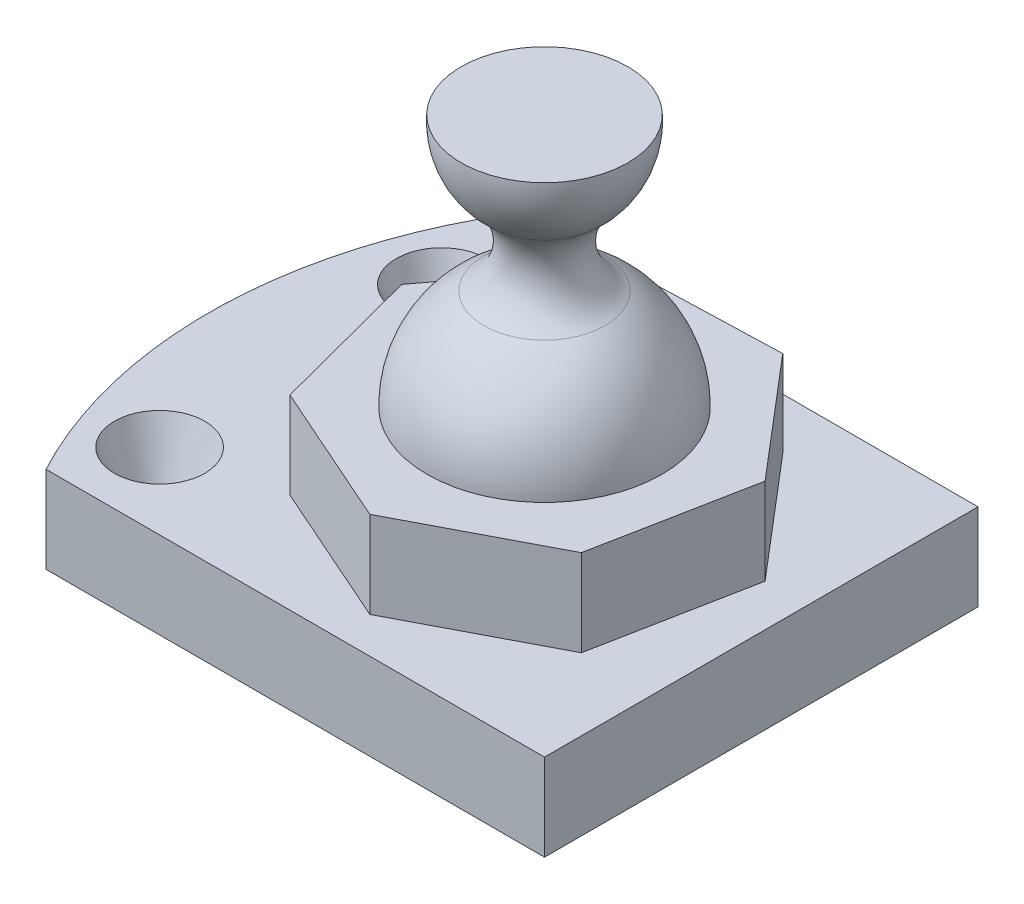
ISO-10303-21;
HEADER;
FILE_DESCRIPTION(('STEP AP214'),'2;1');
FILE_NAME('part.step','',(''),(''),'','','');
FILE_SCHEMA(('AUTOMOTIVE_DESIGN { 1 0 10303 214 1 1 1 1 }'));
ENDSEC;
DATA;
#1=APPLICATION_CONTEXT('core data for automotive mechanical design processes');
#2=APPLICATION_PROTOCOL_DEFINITION('international standard','automotive_design',2000,#1);
#3=PRODUCT_CONTEXT('',#1,'mechanical');
#4=PRODUCT('Part','Part','',(#3));
#5=PRODUCT_RELATED_PRODUCT_CATEGORY('part','',(#4));
#6=PRODUCT_DEFINITION_FORMATION('','',#4);
#7=PRODUCT_DEFINITION_CONTEXT('part definition',#1,'design');
#8=PRODUCT_DEFINITION('design','',#6,#7);
#9=PRODUCT_DEFINITION_SHAPE('','',#8);
#10=(LENGTH_UNIT() NAMED_UNIT(*) SI_UNIT(.MILLI.,.METRE.));
#11=(NAMED_UNIT(*) PLANE_ANGLE_UNIT() SI_UNIT($,.RADIAN.));
#12=(NAMED_UNIT(*) SI_UNIT($,.STERADIAN.) SOLID_ANGLE_UNIT());
#13=UNCERTAINTY_MEASURE_WITH_UNIT(LENGTH_MEASURE(1.E-05),#10,'distance_accuracy_value','');
#14=(GEOMETRIC_REPRESENTATION_CONTEXT(3) GLOBAL_UNCERTAINTY_ASSIGNED_CONTEXT((#13)) GLOBAL_UNIT_ASSIGNED_CONTEXT((#10,
#11,#12)) REPRESENTATION_CONTEXT('',''));
#15=CARTESIAN_POINT('',(0.,0.,0.));
#16=DIRECTION('',(0.,0.,1.));
#17=DIRECTION('',(1.,0.,0.));
#18=AXIS2_PLACEMENT_3D('',#15,#16,#17);
#19=CARTESIAN_POINT('',(0.,0.,0.));
#20=DIRECTION('',(0.,-1.,0.));
#21=DIRECTION('',(1.,0.,0.));
#22=AXIS2_PLACEMENT_3D('',#19,#20,#21);
#23=SPHERICAL_SURFACE('',#22,32.4762304839796);
#24=CARTESIAN_POINT('',(0.,27.8110758941161,0.));
#25=DIRECTION('',(0.,-1.,0.));
#26=DIRECTION('',(0.,0.,-1.));
#27=AXIS2_PLACEMENT_3D('',#24,#25,#26);
#28=CIRCLE('',#27,16.7704980266027);
#29=CARTESIAN_POINT('',(0.,27.8110758941161,-16.7704980266027));
#30=VERTEX_POINT('',#29);
#31=EDGE_CURVE('E172',#30,#30,#28,.T.);
#32=ORIENTED_EDGE('',*,*,#31,.T.);
#33=EDGE_LOOP('',(#32));
#34=FACE_BOUND('',#33,.T.);
#35=CARTESIAN_POINT('',(0.,0.,0.));
#36=DIRECTION('',(0.,-1.,0.));
#37=DIRECTION('',(0.,0.,-1.));
#38=AXIS2_PLACEMENT_3D('',#35,#36,#37);
#39=CIRCLE('',#38,32.4762304839796);
#40=CARTESIAN_POINT('',(0.,0.,-32.4762304839796));
#41=VERTEX_POINT('',#40);
#42=EDGE_CURVE('E49',#41,#41,#39,.T.);
#43=ORIENTED_EDGE('',*,*,#42,.F.);
#44=EDGE_LOOP('',(#43));
#45=FACE_BOUND('',#44,.T.);
#46=ADVANCED_FACE('F37',(#34,#45),#23,.T.);
#47=CARTESIAN_POINT('',(0.,39.8,0.));
#48=DIRECTION('',(0.,-1.,0.));
#49=DIRECTION('',(0.,0.,-1.));
#50=AXIS2_PLACEMENT_3D('',#47,#48,#49);
#51=TOROIDAL_SURFACE('',#50,24.,14.);
#52=CARTESIAN_POINT('',(0.,50.3791238896694,0.));
#53=DIRECTION('',(0.,-1.,0.));
#54=DIRECTION('',(0.,0.,-1.));
#55=AXIS2_PLACEMENT_3D('',#52,#53,#54);
#56=CIRCLE('',#55,14.8303687245873);
#57=CARTESIAN_POINT('',(0.,50.3791238896694,-14.8303687245873));
#58=VERTEX_POINT('',#57);
#59=EDGE_CURVE('E168',#58,#58,#56,.T.);
#60=ORIENTED_EDGE('',*,*,#59,.T.);
#61=EDGE_LOOP('',(#60));
#62=FACE_BOUND('',#61,.T.);
#63=ORIENTED_EDGE('',*,*,#31,.F.);
#64=EDGE_LOOP('',(#63));
#65=FACE_BOUND('',#64,.T.);
#66=ADVANCED_FACE('F185',(#62,#65),#51,.F.);
#67=CARTESIAN_POINT('',(0.,68.5147648433883,0.));
#68=DIRECTION('',(0.,-1.,0.));
#69=DIRECTION('',(0.,0.,-1.));
#70=AXIS2_PLACEMENT_3D('',#67,#68,#69);
#71=DEGENERATE_TOROIDAL_SURFACE('',#70,0.888999176120141,24.,.F.);
#72=CARTESIAN_POINT('',(0.,70.,0.));
#73=DIRECTION('',(0.,-1.,0.));
#74=DIRECTION('',(0.,0.,-1.));
#75=AXIS2_PLACEMENT_3D('',#72,#73,#74);
#76=CIRCLE('',#75,23.065);
#77=CARTESIAN_POINT('',(0.,70.,-23.065));
#78=VERTEX_POINT('',#77);
#79=EDGE_CURVE('E170',#78,#78,#76,.T.);
#80=ORIENTED_EDGE('',*,*,#79,.T.);
#81=EDGE_LOOP('',(#80));
#82=FACE_BOUND('',#81,.T.);
#83=ORIENTED_EDGE('',*,*,#59,.F.);
#84=EDGE_LOOP('',(#83));
#85=FACE_BOUND('',#84,.T.);
#86=ADVANCED_FACE('F189',(#82,#85),#71,.F.);
#87=CARTESIAN_POINT('',(0.,70.,0.));
#88=DIRECTION('',(0.,1.,0.));
#89=DIRECTION('',(0.,0.,1.));
#90=AXIS2_PLACEMENT_3D('',#87,#88,#89);
#91=PLANE('',#90);
#92=ORIENTED_EDGE('',*,*,#79,.F.);
#93=EDGE_LOOP('',(#92));
#94=FACE_BOUND('',#93,.T.);
#95=ADVANCED_FACE('F195',(#94),#91,.T.);
#96=CARTESIAN_POINT('',(0.,0.,0.));
#97=DIRECTION('',(0.,-1.,0.));
#98=DIRECTION('',(0.,0.,-1.));
#99=AXIS2_PLACEMENT_3D('',#96,#97,#98);
#100=PLANE('',#99);
#101=ORIENTED_EDGE('',*,*,#42,.T.);
#102=EDGE_LOOP('',(#101));
#103=FACE_BOUND('',#102,.T.);
#104=DIRECTION('',(-0.886439698937166,0.,0.462844099182637));
#105=VECTOR('',#104,1.);
#106=CARTESIAN_POINT('',(40.0809947566498,0.,29.8917021816659));
#107=LINE('',#106,#105);
#108=CARTESIAN_POINT('',(40.0809947566498,0.,29.8917021816659));
#109=VERTEX_POINT('',#108);
#110=CARTESIAN_POINT('',(1.61981764893979,0.,49.973755019852));
#111=VERTEX_POINT('',#110);
#112=EDGE_CURVE('E145',#109,#111,#107,.T.);
#113=ORIENTED_EDGE('',*,*,#112,.F.);
#114=DIRECTION('',(-0.190820024034508,0.,0.981625039629425));
#115=VECTOR('',#114,1.);
#116=CARTESIAN_POINT('',(48.3603653093092,0.,-12.6994120789177));
#117=LINE('',#116,#115);
#118=CARTESIAN_POINT('',(48.3603653093092,0.,-12.6994120789177));
#119=VERTEX_POINT('',#118);
#120=EDGE_CURVE('E90',#119,#109,#117,.T.);
#121=ORIENTED_EDGE('',*,*,#120,.F.);
#122=DIRECTION('',(0.648491020985258,0.,0.761222303733606));
#123=VECTOR('',#122,1.);
#124=CARTESIAN_POINT('',(20.2233944123846,0.,-45.7276100232795));
#125=LINE('',#124,#123);
#126=CARTESIAN_POINT('',(20.2233944123846,0.,-45.7276100232795));
#127=VERTEX_POINT('',#126);
#128=EDGE_CURVE('E85',#127,#119,#125,.T.);
#129=ORIENTED_EDGE('',*,*,#128,.F.);
#130=DIRECTION('',(0.99947510039704,0.,-0.0323963529787958));
#131=VECTOR('',#130,1.);
#132=CARTESIAN_POINT('',(-23.1422049591319,0.,-44.3219849468583));
#133=LINE('',#132,#131);
#134=CARTESIAN_POINT('',(-23.1422049591319,0.,-44.3219849468583));
#135=VERTEX_POINT('',#134);
#136=EDGE_CURVE('E153',#135,#127,#133,.T.);
#137=ORIENTED_EDGE('',*,*,#136,.F.);
#138=DIRECTION('',(0.597834043633319,0.,-0.801619895132996));
#139=VECTOR('',#138,1.);
#140=CARTESIAN_POINT('',(-49.0812519814712,0.,-9.54100120172539));
#141=LINE('',#140,#139);
#142=CARTESIAN_POINT('',(-49.0812519814712,0.,-9.54100120172539));
#143=VERTEX_POINT('',#142);
#144=EDGE_CURVE('E117',#143,#135,#141,.T.);
#145=ORIENTED_EDGE('',*,*,#144,.F.);
#146=DIRECTION('',(-0.253988241578353,0.,-0.967207306186185));
#147=VECTOR('',#146,1.);
#148=CARTESIAN_POINT('',(-38.0611151866803,0.,32.4245510492629));
#149=LINE('',#148,#147);
#150=CARTESIAN_POINT('',(-38.0611151866803,0.,32.4245510492629));
#151=VERTEX_POINT('',#150);
#152=EDGE_CURVE('E147',#151,#143,#149,.T.);
#153=ORIENTED_EDGE('',*,*,#152,.F.);
#154=DIRECTION('',(-0.91455220046559,0.,-0.404467888247692));
#155=VECTOR('',#154,1.);
#156=CARTESIAN_POINT('',(1.61981764893979,0.,49.973755019852));
#157=LINE('',#156,#155);
#158=EDGE_CURVE('E150',#111,#151,#157,.T.);
#159=ORIENTED_EDGE('',*,*,#158,.F.);
#160=EDGE_LOOP('',(#113,#121,#129,#137,#145,#153,#159));
#161=FACE_BOUND('',#160,.T.);
#162=ADVANCED_FACE('F180',(#103,#161),#100,.F.);
#163=CARTESIAN_POINT('',(40.0809947566498,-24.,29.8917021816659));
#164=DIRECTION('',(-0.462844099182637,0.,-0.886439698937166));
#165=DIRECTION('',(-0.886439698937166,0.,0.462844099182637));
#166=AXIS2_PLACEMENT_3D('',#163,#164,#165);
#167=PLANE('',#166);
#168=ORIENTED_EDGE('',*,*,#112,.T.);
#169=DIRECTION('',(0.,1.,0.));
#170=VECTOR('',#169,1.);
#171=CARTESIAN_POINT('',(1.61981764893979,-24.,49.973755019852));
#172=LINE('',#171,#170);
#173=CARTESIAN_POINT('',(1.61981764893979,-24.,49.973755019852));
#174=VERTEX_POINT('',#173);
#175=EDGE_CURVE('E164',#174,#111,#172,.T.);
#176=ORIENTED_EDGE('',*,*,#175,.F.);
#177=DIRECTION('',(-0.886439698937166,0.,0.462844099182637));
#178=VECTOR('',#177,1.);
#179=CARTESIAN_POINT('',(40.0809947566498,-24.,29.8917021816659));
#180=LINE('',#179,#178);
#181=CARTESIAN_POINT('',(40.0809947566498,-24.,29.8917021816659));
#182=VERTEX_POINT('',#181);
#183=EDGE_CURVE('E160',#182,#174,#180,.T.);
#184=ORIENTED_EDGE('',*,*,#183,.F.);
#185=DIRECTION('',(0.,1.,0.));
#186=VECTOR('',#185,1.);
#187=CARTESIAN_POINT('',(40.0809947566498,-24.,29.8917021816659));
#188=LINE('',#187,#186);
#189=EDGE_CURVE('E141',#182,#109,#188,.T.);
#190=ORIENTED_EDGE('',*,*,#189,.T.);
#191=EDGE_LOOP('',(#168,#176,#184,#190));
#192=FACE_BOUND('',#191,.T.);
#193=ADVANCED_FACE('F196',(#192),#167,.F.);
#194=CARTESIAN_POINT('',(1.61981764893979,-24.,49.973755019852));
#195=DIRECTION('',(0.404467888247692,0.,-0.91455220046559));
#196=DIRECTION('',(-0.91455220046559,0.,-0.404467888247692));
#197=AXIS2_PLACEMENT_3D('',#194,#195,#196);
#198=PLANE('',#197);
#199=ORIENTED_EDGE('',*,*,#158,.T.);
#200=DIRECTION('',(0.,1.,0.));
#201=VECTOR('',#200,1.);
#202=CARTESIAN_POINT('',(-38.0611151866803,-24.,32.4245510492629));
#203=LINE('',#202,#201);
#204=CARTESIAN_POINT('',(-38.0611151866803,-24.,32.4245510492629));
#205=VERTEX_POINT('',#204);
#206=EDGE_CURVE('E165',#205,#151,#203,.T.);
#207=ORIENTED_EDGE('',*,*,#206,.F.);
#208=DIRECTION('',(-0.91455220046559,0.,-0.404467888247692));
#209=VECTOR('',#208,1.);
#210=CARTESIAN_POINT('',(1.61981764893979,-24.,49.973755019852));
#211=LINE('',#210,#209);
#212=EDGE_CURVE('E98',#174,#205,#211,.T.);
#213=ORIENTED_EDGE('',*,*,#212,.F.);
#214=ORIENTED_EDGE('',*,*,#175,.T.);
#215=EDGE_LOOP('',(#199,#207,#213,#214));
#216=FACE_BOUND('',#215,.T.);
#217=ADVANCED_FACE('F203',(#216),#198,.F.);
#218=CARTESIAN_POINT('',(-38.0611151866803,-24.,32.4245510492629));
#219=DIRECTION('',(0.967207306186185,0.,-0.253988241578353));
#220=DIRECTION('',(-0.253988241578353,0.,-0.967207306186185));
#221=AXIS2_PLACEMENT_3D('',#218,#219,#220);
#222=PLANE('',#221);
#223=ORIENTED_EDGE('',*,*,#152,.T.);
#224=DIRECTION('',(0.,1.,0.));
#225=VECTOR('',#224,1.);
#226=CARTESIAN_POINT('',(-49.0812519814712,-24.,-9.54100120172539));
#227=LINE('',#226,#225);
#228=CARTESIAN_POINT('',(-49.0812519814712,-24.,-9.54100120172539));
#229=VERTEX_POINT('',#228);
#230=EDGE_CURVE('E124',#229,#143,#227,.T.);
#231=ORIENTED_EDGE('',*,*,#230,.F.);
#232=DIRECTION('',(-0.253988241578353,0.,-0.967207306186185));
#233=VECTOR('',#232,1.);
#234=CARTESIAN_POINT('',(-38.0611151866803,-24.,32.4245510492629));
#235=LINE('',#234,#233);
#236=EDGE_CURVE('E131',#205,#229,#235,.T.);
#237=ORIENTED_EDGE('',*,*,#236,.F.);
#238=ORIENTED_EDGE('',*,*,#206,.T.);
#239=EDGE_LOOP('',(#223,#231,#237,#238));
#240=FACE_BOUND('',#239,.T.);
#241=ADVANCED_FACE('F202',(#240),#222,.F.);
#242=CARTESIAN_POINT('',(-49.0812519814712,-24.,-9.54100120172539));
#243=DIRECTION('',(0.801619895132996,0.,0.597834043633319));
#244=DIRECTION('',(0.597834043633319,0.,-0.801619895132996));
#245=AXIS2_PLACEMENT_3D('',#242,#243,#244);
#246=PLANE('',#245);
#247=ORIENTED_EDGE('',*,*,#144,.T.);
#248=DIRECTION('',(0.,1.,0.));
#249=VECTOR('',#248,1.);
#250=CARTESIAN_POINT('',(-23.1422049591319,-24.,-44.3219849468583));
#251=LINE('',#250,#249);
#252=CARTESIAN_POINT('',(-23.1422049591319,-24.,-44.3219849468583));
#253=VERTEX_POINT('',#252);
#254=EDGE_CURVE('E109',#253,#135,#251,.T.);
#255=ORIENTED_EDGE('',*,*,#254,.F.);
#256=DIRECTION('',(0.597834043633319,0.,-0.801619895132996));
#257=VECTOR('',#256,1.);
#258=CARTESIAN_POINT('',(-49.0812519814712,-24.,-9.54100120172539));
#259=LINE('',#258,#257);
#260=EDGE_CURVE('E113',#229,#253,#259,.T.);
#261=ORIENTED_EDGE('',*,*,#260,.F.);
#262=ORIENTED_EDGE('',*,*,#230,.T.);
#263=EDGE_LOOP('',(#247,#255,#261,#262));
#264=FACE_BOUND('',#263,.T.);
#265=ADVANCED_FACE('F115',(#264),#246,.F.);
#266=CARTESIAN_POINT('',(-23.1422049591319,-24.,-44.3219849468583));
#267=DIRECTION('',(0.0323963529787958,0.,0.99947510039704));
#268=DIRECTION('',(0.99947510039704,0.,-0.0323963529787958));
#269=AXIS2_PLACEMENT_3D('',#266,#267,#268);
#270=PLANE('',#269);
#271=ORIENTED_EDGE('',*,*,#136,.T.);
#272=DIRECTION('',(0.,1.,0.));
#273=VECTOR('',#272,1.);
#274=CARTESIAN_POINT('',(20.2233944123846,-24.,-45.7276100232795));
#275=LINE('',#274,#273);
#276=CARTESIAN_POINT('',(20.2233944123846,-24.,-45.7276100232795));
#277=VERTEX_POINT('',#276);
#278=EDGE_CURVE('E121',#277,#127,#275,.T.);
#279=ORIENTED_EDGE('',*,*,#278,.F.);
#280=DIRECTION('',(0.99947510039704,0.,-0.0323963529787958));
#281=VECTOR('',#280,1.);
#282=CARTESIAN_POINT('',(-23.1422049591319,-24.,-44.3219849468583));
#283=LINE('',#282,#281);
#284=EDGE_CURVE('E122',#253,#277,#283,.T.);
#285=ORIENTED_EDGE('',*,*,#284,.F.);
#286=ORIENTED_EDGE('',*,*,#254,.T.);
#287=EDGE_LOOP('',(#271,#279,#285,#286));
#288=FACE_BOUND('',#287,.T.);
#289=ADVANCED_FACE('F127',(#288),#270,.F.);
#290=CARTESIAN_POINT('',(20.2233944123846,-24.,-45.7276100232795));
#291=DIRECTION('',(-0.761222303733606,0.,0.648491020985258));
#292=DIRECTION('',(0.648491020985258,0.,0.761222303733606));
#293=AXIS2_PLACEMENT_3D('',#290,#291,#292);
#294=PLANE('',#293);
#295=ORIENTED_EDGE('',*,*,#128,.T.);
#296=DIRECTION('',(0.,1.,0.));
#297=VECTOR('',#296,1.);
#298=CARTESIAN_POINT('',(48.3603653093092,-24.,-12.6994120789177));
#299=LINE('',#298,#297);
#300=CARTESIAN_POINT('',(48.3603653093092,-24.,-12.6994120789177));
#301=VERTEX_POINT('',#300);
#302=EDGE_CURVE('E59',#301,#119,#299,.T.);
#303=ORIENTED_EDGE('',*,*,#302,.F.);
#304=DIRECTION('',(0.648491020985258,0.,0.761222303733606));
#305=VECTOR('',#304,1.);
#306=CARTESIAN_POINT('',(20.2233944123846,-24.,-45.7276100232795));
#307=LINE('',#306,#305);
#308=EDGE_CURVE('E129',#277,#301,#307,.T.);
#309=ORIENTED_EDGE('',*,*,#308,.F.);
#310=ORIENTED_EDGE('',*,*,#278,.T.);
#311=EDGE_LOOP('',(#295,#303,#309,#310));
#312=FACE_BOUND('',#311,.T.);
#313=ADVANCED_FACE('F213',(#312),#294,.F.);
#314=CARTESIAN_POINT('',(48.3603653093092,-24.,-12.6994120789177));
#315=DIRECTION('',(-0.981625039629425,0.,-0.190820024034508));
#316=DIRECTION('',(-0.190820024034508,0.,0.981625039629425));
#317=AXIS2_PLACEMENT_3D('',#314,#315,#316);
#318=PLANE('',#317);
#319=ORIENTED_EDGE('',*,*,#120,.T.);
#320=ORIENTED_EDGE('',*,*,#189,.F.);
#321=DIRECTION('',(-0.190820024034508,0.,0.981625039629425));
#322=VECTOR('',#321,1.);
#323=CARTESIAN_POINT('',(48.3603653093092,-24.,-12.6994120789177));
#324=LINE('',#323,#322);
#325=EDGE_CURVE('E143',#301,#182,#324,.T.);
#326=ORIENTED_EDGE('',*,*,#325,.F.);
#327=ORIENTED_EDGE('',*,*,#302,.T.);
#328=EDGE_LOOP('',(#319,#320,#326,#327));
#329=FACE_BOUND('',#328,.T.);
#330=ADVANCED_FACE('F216',(#329),#318,.F.);
#331=CARTESIAN_POINT('',(60.,-48.,60.));
#332=DIRECTION('',(-1.,0.,0.));
#333=DIRECTION('',(0.,0.,1.));
#334=AXIS2_PLACEMENT_3D('',#331,#332,#333);
#335=PLANE('',#334);
#336=DIRECTION('',(0.,0.,1.));
#337=VECTOR('',#336,1.);
#338=CARTESIAN_POINT('',(60.,-24.,60.));
#339=LINE('',#338,#337);
#340=CARTESIAN_POINT('',(60.,-24.,-60.));
#341=VERTEX_POINT('',#340);
#342=CARTESIAN_POINT('',(60.,-24.,60.));
#343=VERTEX_POINT('',#342);
#344=EDGE_CURVE('E268',#341,#343,#339,.T.);
#345=ORIENTED_EDGE('',*,*,#344,.T.);
#346=DIRECTION('',(0.,1.,0.));
#347=VECTOR('',#346,1.);
#348=CARTESIAN_POINT('',(60.,-48.,60.));
#349=LINE('',#348,#347);
#350=CARTESIAN_POINT('',(60.,-48.,60.));
#351=VERTEX_POINT('',#350);
#352=EDGE_CURVE('E306',#351,#343,#349,.T.);
#353=ORIENTED_EDGE('',*,*,#352,.F.);
#354=DIRECTION('',(0.,0.,1.));
#355=VECTOR('',#354,1.);
#356=CARTESIAN_POINT('',(60.,-48.,60.));
#357=LINE('',#356,#355);
#358=CARTESIAN_POINT('',(60.,-48.,-60.));
#359=VERTEX_POINT('',#358);
#360=EDGE_CURVE('E277',#359,#351,#357,.T.);
#361=ORIENTED_EDGE('',*,*,#360,.F.);
#362=DIRECTION('',(0.,1.,0.));
#363=VECTOR('',#362,1.);
#364=CARTESIAN_POINT('',(60.,-48.,-60.));
#365=LINE('',#364,#363);
#366=EDGE_CURVE('E288',#359,#341,#365,.T.);
#367=ORIENTED_EDGE('',*,*,#366,.T.);
#368=EDGE_LOOP('',(#345,#353,#361,#367));
#369=FACE_BOUND('',#368,.T.);
#370=ADVANCED_FACE('F218',(#369),#335,.F.);
#371=CARTESIAN_POINT('',(-78.,-48.,60.));
#372=DIRECTION('',(0.,0.,-1.));
#373=DIRECTION('',(-1.,0.,0.));
#374=AXIS2_PLACEMENT_3D('',#371,#372,#373);
#375=PLANE('',#374);
#376=DIRECTION('',(-1.,0.,0.));
#377=VECTOR('',#376,1.);
#378=CARTESIAN_POINT('',(-78.,-24.,60.));
#379=LINE('',#378,#377);
#380=CARTESIAN_POINT('',(-78.,-24.,60.));
#381=VERTEX_POINT('',#380);
#382=EDGE_CURVE('E295',#343,#381,#379,.T.);
#383=ORIENTED_EDGE('',*,*,#382,.T.);
#384=DIRECTION('',(0.,1.,0.));
#385=VECTOR('',#384,1.);
#386=CARTESIAN_POINT('',(-78.,-48.,60.));
#387=LINE('',#386,#385);
#388=CARTESIAN_POINT('',(-78.,-48.,60.));
#389=VERTEX_POINT('',#388);
#390=EDGE_CURVE('E302',#389,#381,#387,.T.);
#391=ORIENTED_EDGE('',*,*,#390,.F.);
#392=DIRECTION('',(-1.,0.,0.));
#393=VECTOR('',#392,1.);
#394=CARTESIAN_POINT('',(-78.,-48.,60.));
#395=LINE('',#394,#393);
#396=EDGE_CURVE('E276',#351,#389,#395,.T.);
#397=ORIENTED_EDGE('',*,*,#396,.F.);
#398=ORIENTED_EDGE('',*,*,#352,.T.);
#399=EDGE_LOOP('',(#383,#391,#397,#398));
#400=FACE_BOUND('',#399,.T.);
#401=ADVANCED_FACE('F226',(#400),#375,.F.);
#402=CARTESIAN_POINT('',(34.5,-48.,0.));
#403=DIRECTION('',(0.,1.,0.));
#404=DIRECTION('',(0.,0.,1.));
#405=AXIS2_PLACEMENT_3D('',#402,#403,#404);
#406=CYLINDRICAL_SURFACE('',#405,127.5);
#407=CARTESIAN_POINT('',(34.5,-24.,0.));
#408=DIRECTION('',(0.,-1.,0.));
#409=DIRECTION('',(0.,0.,1.));
#410=AXIS2_PLACEMENT_3D('',#407,#408,#409);
#411=CIRCLE('',#410,127.5);
#412=CARTESIAN_POINT('',(-78.,-24.,-60.));
#413=VERTEX_POINT('',#412);
#414=EDGE_CURVE('E293',#381,#413,#411,.T.);
#415=ORIENTED_EDGE('',*,*,#414,.T.);
#416=DIRECTION('',(0.,1.,0.));
#417=VECTOR('',#416,1.);
#418=CARTESIAN_POINT('',(-78.,-48.,-60.));
#419=LINE('',#418,#417);
#420=CARTESIAN_POINT('',(-78.,-48.,-60.));
#421=VERTEX_POINT('',#420);
#422=EDGE_CURVE('E301',#421,#413,#419,.T.);
#423=ORIENTED_EDGE('',*,*,#422,.F.);
#424=CARTESIAN_POINT('',(34.5,-48.,0.));
#425=DIRECTION('',(0.,-1.,0.));
#426=DIRECTION('',(0.,0.,1.));
#427=AXIS2_PLACEMENT_3D('',#424,#425,#426);
#428=CIRCLE('',#427,127.5);
#429=EDGE_CURVE('E282',#389,#421,#428,.T.);
#430=ORIENTED_EDGE('',*,*,#429,.F.);
#431=ORIENTED_EDGE('',*,*,#390,.T.);
#432=EDGE_LOOP('',(#415,#423,#430,#431));
#433=FACE_BOUND('',#432,.T.);
#434=ADVANCED_FACE('F233',(#433),#406,.T.);
#435=CARTESIAN_POINT('',(60.,-48.,-60.));
#436=DIRECTION('',(0.,0.,1.));
#437=DIRECTION('',(1.,0.,0.));
#438=AXIS2_PLACEMENT_3D('',#435,#436,#437);
#439=PLANE('',#438);
#440=DIRECTION('',(1.,0.,0.));
#441=VECTOR('',#440,1.);
#442=CARTESIAN_POINT('',(60.,-24.,-60.));
#443=LINE('',#442,#441);
#444=EDGE_CURVE('E278',#413,#341,#443,.T.);
#445=ORIENTED_EDGE('',*,*,#444,.T.);
#446=ORIENTED_EDGE('',*,*,#366,.F.);
#447=DIRECTION('',(1.,0.,0.));
#448=VECTOR('',#447,1.);
#449=CARTESIAN_POINT('',(60.,-48.,-60.));
#450=LINE('',#449,#448);
#451=EDGE_CURVE('E289',#421,#359,#450,.T.);
#452=ORIENTED_EDGE('',*,*,#451,.F.);
#453=ORIENTED_EDGE('',*,*,#422,.T.);
#454=EDGE_LOOP('',(#445,#446,#452,#453));
#455=FACE_BOUND('',#454,.T.);
#456=ADVANCED_FACE('F236',(#455),#439,.F.);
#457=CARTESIAN_POINT('',(34.5,-48.,0.));
#458=DIRECTION('',(0.,1.,0.));
#459=DIRECTION('',(0.,0.,1.));
#460=AXIS2_PLACEMENT_3D('',#457,#458,#459);
#461=PLANE('',#460);
#462=CARTESIAN_POINT('',(-67.55,-48.,-39.));
#463=DIRECTION('',(0.,1.,0.));
#464=DIRECTION('',(0.,0.,1.));
#465=AXIS2_PLACEMENT_3D('',#462,#463,#464);
#466=CIRCLE('',#465,3.76471437761112);
#467=CARTESIAN_POINT('',(-67.55,-48.,-35.2352856223889));
#468=VERTEX_POINT('',#467);
#469=EDGE_CURVE('E265',#468,#468,#466,.F.);
#470=ORIENTED_EDGE('',*,*,#469,.F.);
#471=EDGE_LOOP('',(#470));
#472=FACE_BOUND('',#471,.T.);
#473=CARTESIAN_POINT('',(-67.55,-48.,39.));
#474=DIRECTION('',(0.,1.,0.));
#475=DIRECTION('',(0.,0.,1.));
#476=AXIS2_PLACEMENT_3D('',#473,#474,#475);
#477=CIRCLE('',#476,3.76471437761112);
#478=CARTESIAN_POINT('',(-67.55,-48.,42.7647143776111));
#479=VERTEX_POINT('',#478);
#480=EDGE_CURVE('E271',#479,#479,#477,.F.);
#481=ORIENTED_EDGE('',*,*,#480,.F.);
#482=EDGE_LOOP('',(#481));
#483=FACE_BOUND('',#482,.T.);
#484=ORIENTED_EDGE('',*,*,#360,.T.);
#485=ORIENTED_EDGE('',*,*,#396,.T.);
#486=ORIENTED_EDGE('',*,*,#429,.T.);
#487=ORIENTED_EDGE('',*,*,#451,.T.);
#488=EDGE_LOOP('',(#484,#485,#486,#487));
#489=FACE_BOUND('',#488,.T.);
#490=ADVANCED_FACE('F244',(#472,#483,#489),#461,.F.);
#491=CARTESIAN_POINT('',(34.5,-24.,0.));
#492=DIRECTION('',(0.,1.,0.));
#493=DIRECTION('',(0.,0.,1.));
#494=AXIS2_PLACEMENT_3D('',#491,#492,#493);
#495=PLANE('',#494);
#496=CARTESIAN_POINT('',(-67.55,-24.,-39.));
#497=DIRECTION('',(0.,1.,0.));
#498=DIRECTION('',(0.,0.,1.));
#499=AXIS2_PLACEMENT_3D('',#496,#497,#498);
#500=CIRCLE('',#499,12.5);
#501=CARTESIAN_POINT('',(-67.55,-24.,-26.5));
#502=VERTEX_POINT('',#501);
#503=EDGE_CURVE('E264',#502,#502,#500,.T.);
#504=ORIENTED_EDGE('',*,*,#503,.F.);
#505=EDGE_LOOP('',(#504));
#506=FACE_BOUND('',#505,.T.);
#507=CARTESIAN_POINT('',(-67.55,-24.,39.));
#508=DIRECTION('',(0.,1.,0.));
#509=DIRECTION('',(0.,0.,1.));
#510=AXIS2_PLACEMENT_3D('',#507,#508,#509);
#511=CIRCLE('',#510,12.5);
#512=CARTESIAN_POINT('',(-67.55,-24.,51.5));
#513=VERTEX_POINT('',#512);
#514=EDGE_CURVE('E266',#513,#513,#511,.T.);
#515=ORIENTED_EDGE('',*,*,#514,.F.);
#516=EDGE_LOOP('',(#515));
#517=FACE_BOUND('',#516,.T.);
#518=ORIENTED_EDGE('',*,*,#325,.T.);
#519=ORIENTED_EDGE('',*,*,#183,.T.);
#520=ORIENTED_EDGE('',*,*,#212,.T.);
#521=ORIENTED_EDGE('',*,*,#236,.T.);
#522=ORIENTED_EDGE('',*,*,#260,.T.);
#523=ORIENTED_EDGE('',*,*,#284,.T.);
#524=ORIENTED_EDGE('',*,*,#308,.T.);
#525=EDGE_LOOP('',(#518,#519,#520,#521,#522,#523,#524));
#526=FACE_BOUND('',#525,.T.);
#527=ORIENTED_EDGE('',*,*,#344,.F.);
#528=ORIENTED_EDGE('',*,*,#444,.F.);
#529=ORIENTED_EDGE('',*,*,#414,.F.);
#530=ORIENTED_EDGE('',*,*,#382,.F.);
#531=EDGE_LOOP('',(#527,#528,#529,#530));
#532=FACE_BOUND('',#531,.T.);
#533=ADVANCED_FACE('F134',(#506,#517,#526,#532),#495,.T.);
#534=CARTESIAN_POINT('',(-67.55,-24.,39.));
#535=DIRECTION('',(0.,1.,0.));
#536=DIRECTION('',(0.,0.,1.));
#537=AXIS2_PLACEMENT_3D('',#534,#535,#536);
#538=CONICAL_SURFACE('',#537,12.5,0.349065850398867);
#539=CARTESIAN_POINT('',(-67.55,-48.,42.7647143776111));
#540=CARTESIAN_POINT('',(-67.55,-47.75,42.8557069361777));
#541=CARTESIAN_POINT('',(-67.55,-47.5,42.9466994947442));
#542=CARTESIAN_POINT('',(-67.55,-47.,43.1286846118773));
#543=CARTESIAN_POINT('',(-67.55,-46.75,43.2196771704439));
#544=CARTESIAN_POINT('',(-67.55,-46.25,43.401662287577));
#545=CARTESIAN_POINT('',(-67.55,-46.,43.4926548461435));
#546=CARTESIAN_POINT('',(-67.55,-45.5,43.6746399632766));
#547=CARTESIAN_POINT('',(-67.55,-45.25,43.7656325218432));
#548=CARTESIAN_POINT('',(-67.55,-44.75,43.9476176389763));
#549=CARTESIAN_POINT('',(-67.55,-44.5,44.0386101975428));
#550=CARTESIAN_POINT('',(-67.55,-44.,44.2205953146759));
#551=CARTESIAN_POINT('',(-67.55,-43.75,44.3115878732425));
#552=CARTESIAN_POINT('',(-67.55,-43.25,44.4935729903756));
#553=CARTESIAN_POINT('',(-67.55,-43.,44.5845655489421));
#554=CARTESIAN_POINT('',(-67.55,-42.5,44.7665506660752));
#555=CARTESIAN_POINT('',(-67.55,-42.25,44.8575432246418));
#556=CARTESIAN_POINT('',(-67.55,-41.75,45.0395283417749));
#557=CARTESIAN_POINT('',(-67.55,-41.5,45.1305209003414));
#558=CARTESIAN_POINT('',(-67.55,-41.,45.3125060174745));
#559=CARTESIAN_POINT('',(-67.55,-40.75,45.4034985760411));
#560=CARTESIAN_POINT('',(-67.55,-40.25,45.5854836931742));
#561=CARTESIAN_POINT('',(-67.55,-40.,45.6764762517407));
#562=CARTESIAN_POINT('',(-67.55,-39.5,45.8584613688738));
#563=CARTESIAN_POINT('',(-67.55,-39.25,45.9494539274404));
#564=CARTESIAN_POINT('',(-67.55,-38.75,46.1314390445735));
#565=CARTESIAN_POINT('',(-67.55,-38.5,46.22243160314));
#566=CARTESIAN_POINT('',(-67.55,-38.,46.4044167202731));
#567=CARTESIAN_POINT('',(-67.55,-37.75,46.4954092788397));
#568=CARTESIAN_POINT('',(-67.55,-37.25,46.6773943959728));
#569=CARTESIAN_POINT('',(-67.55,-37.,46.7683869545394));
#570=CARTESIAN_POINT('',(-67.55,-36.5,46.9503720716725));
#571=CARTESIAN_POINT('',(-67.55,-36.25,47.041364630239));
#572=CARTESIAN_POINT('',(-67.55,-35.75,47.2233497473721));
#573=CARTESIAN_POINT('',(-67.55,-35.5,47.3143423059387));
#574=CARTESIAN_POINT('',(-67.55,-35.,47.4963274230718));
#575=CARTESIAN_POINT('',(-67.55,-34.75,47.5873199816383));
#576=CARTESIAN_POINT('',(-67.55,-34.25,47.7693050987714));
#577=CARTESIAN_POINT('',(-67.55,-34.,47.860297657338));
#578=CARTESIAN_POINT('',(-67.55,-33.5,48.0422827744711));
#579=CARTESIAN_POINT('',(-67.55,-33.25,48.1332753330376));
#580=CARTESIAN_POINT('',(-67.55,-32.75,48.3152604501707));
#581=CARTESIAN_POINT('',(-67.55,-32.5,48.4062530087373));
#582=CARTESIAN_POINT('',(-67.55,-32.,48.5882381258704));
#583=CARTESIAN_POINT('',(-67.55,-31.75,48.6792306844369));
#584=CARTESIAN_POINT('',(-67.55,-31.25,48.86121580157));
#585=CARTESIAN_POINT('',(-67.55,-31.,48.9522083601366));
#586=CARTESIAN_POINT('',(-67.55,-30.5,49.1341934772697));
#587=CARTESIAN_POINT('',(-67.55,-30.25,49.2251860358362));
#588=CARTESIAN_POINT('',(-67.55,-29.75,49.4071711529693));
#589=CARTESIAN_POINT('',(-67.55,-29.5,49.4981637115359));
#590=CARTESIAN_POINT('',(-67.55,-29.,49.680148828669));
#591=CARTESIAN_POINT('',(-67.55,-28.75,49.7711413872355));
#592=CARTESIAN_POINT('',(-67.55,-28.25,49.9531265043686));
#593=CARTESIAN_POINT('',(-67.55,-28.,50.0441190629352));
#594=CARTESIAN_POINT('',(-67.55,-27.5,50.2261041800683));
#595=CARTESIAN_POINT('',(-67.55,-27.25,50.3170967386348));
#596=CARTESIAN_POINT('',(-67.55,-26.75,50.4990818557679));
#597=CARTESIAN_POINT('',(-67.55,-26.5,50.5900744143345));
#598=CARTESIAN_POINT('',(-67.55,-26.,50.7720595314676));
#599=CARTESIAN_POINT('',(-67.55,-25.75,50.8630520900341));
#600=CARTESIAN_POINT('',(-67.55,-25.25,51.0450372071672));
#601=CARTESIAN_POINT('',(-67.55,-25.,51.1360297657338));
#602=CARTESIAN_POINT('',(-67.55,-24.5,51.3180148828669));
#603=CARTESIAN_POINT('',(-67.55,-24.25,51.4090074414335));
#604=CARTESIAN_POINT('',(-67.55,-24.,51.5));
#605=B_SPLINE_CURVE_WITH_KNOTS('',3,(#539,#540,#541,#542,#543,#544,#545,#546,#547,#548,#549,
#550,#551,#552,#553,#554,#555,#556,#557,#558,#559,#560,#561,#562,#563,#564,#565,#566,#567,#568,
#569,#570,#571,#572,#573,#574,#575,#576,#577,#578,#579,#580,#581,#582,#583,#584,#585,#586,#587,
#588,#589,#590,#591,#592,#593,#594,#595,#596,#597,#598,#599,#600,#601,#602,#603,#604),
.UNSPECIFIED.,.F.,.F.,(4,2,2,2,2,2,2,2,2,2,2,2,2,2,2,2,2,2,2,2,2,2,2,2,2,2,2,2,2,2,2,2,4),(0.,
0.798133329356934,1.59626665871387,2.3943999880708,3.19253331742773,3.99066664678467,
4.7887999761416,5.58693330549854,6.38506663485547,7.18319996421241,7.98133329356934,
8.77946662292628,9.57759995228321,10.3757332816401,11.1738666109971,11.971999940354,
12.770133269711,13.5682665990679,14.3663999284248,15.1645332577818,15.9626665871387,
16.7607999164956,17.5589332458526,18.3570665752095,19.1551999045664,19.9533332339234,
20.7514665632803,21.5495998926372,22.3477332219942,23.1458665513511,23.943999880708,
24.742133210065,25.5402665394219),.UNSPECIFIED.);
#606=EDGE_CURVE('BSEAM249',#479,#513,#605,.T.);
#607=ORIENTED_EDGE('',*,*,#480,.T.);
#608=ORIENTED_EDGE('',*,*,#514,.T.);
#609=ORIENTED_EDGE('',*,*,#606,.T.);
#610=ORIENTED_EDGE('',*,*,#606,.F.);
#611=EDGE_LOOP('',(#607,#609,#608,#610));
#612=FACE_BOUND('',#611,.T.);
#613=ADVANCED_FACE('F249',(#612),#538,.F.);
#614=CARTESIAN_POINT('',(-67.55,-24.,-39.));
#615=DIRECTION('',(0.,1.,0.));
#616=DIRECTION('',(0.,0.,1.));
#617=AXIS2_PLACEMENT_3D('',#614,#615,#616);
#618=CONICAL_SURFACE('',#617,12.5,0.349065850398867);
#619=CARTESIAN_POINT('',(-67.55,-48.,-35.2352856223889));
#620=CARTESIAN_POINT('',(-67.55,-47.75,-35.1442930638223));
#621=CARTESIAN_POINT('',(-67.55,-47.5,-35.0533005052558));
#622=CARTESIAN_POINT('',(-67.55,-47.,-34.8713153881227));
#623=CARTESIAN_POINT('',(-67.55,-46.75,-34.7803228295561));
#624=CARTESIAN_POINT('',(-67.55,-46.25,-34.598337712423));
#625=CARTESIAN_POINT('',(-67.55,-46.,-34.5073451538565));
#626=CARTESIAN_POINT('',(-67.55,-45.5,-34.3253600367234));
#627=CARTESIAN_POINT('',(-67.55,-45.25,-34.2343674781568));
#628=CARTESIAN_POINT('',(-67.55,-44.75,-34.0523823610237));
#629=CARTESIAN_POINT('',(-67.55,-44.5,-33.9613898024572));
#630=CARTESIAN_POINT('',(-67.55,-44.,-33.7794046853241));
#631=CARTESIAN_POINT('',(-67.55,-43.75,-33.6884121267575));
#632=CARTESIAN_POINT('',(-67.55,-43.25,-33.5064270096244));
#633=CARTESIAN_POINT('',(-67.55,-43.,-33.4154344510579));
#634=CARTESIAN_POINT('',(-67.55,-42.5,-33.2334493339248));
#635=CARTESIAN_POINT('',(-67.55,-42.25,-33.1424567753582));
#636=CARTESIAN_POINT('',(-67.55,-41.75,-32.9604716582251));
#637=CARTESIAN_POINT('',(-67.55,-41.5,-32.8694790996586));
#638=CARTESIAN_POINT('',(-67.55,-41.,-32.6874939825255));
#639=CARTESIAN_POINT('',(-67.55,-40.75,-32.5965014239589));
#640=CARTESIAN_POINT('',(-67.55,-40.25,-32.4145163068258));
#641=CARTESIAN_POINT('',(-67.55,-40.,-32.3235237482593));
#642=CARTESIAN_POINT('',(-67.55,-39.5,-32.1415386311262));
#643=CARTESIAN_POINT('',(-67.55,-39.25,-32.0505460725596));
#644=CARTESIAN_POINT('',(-67.55,-38.75,-31.8685609554265));
#645=CARTESIAN_POINT('',(-67.55,-38.5,-31.77756839686));
#646=CARTESIAN_POINT('',(-67.55,-38.,-31.5955832797268));
#647=CARTESIAN_POINT('',(-67.55,-37.75,-31.5045907211603));
#648=CARTESIAN_POINT('',(-67.55,-37.25,-31.3226056040272));
#649=CARTESIAN_POINT('',(-67.55,-37.,-31.2316130454606));
#650=CARTESIAN_POINT('',(-67.55,-36.5,-31.0496279283275));
#651=CARTESIAN_POINT('',(-67.55,-36.25,-30.958635369761));
#652=CARTESIAN_POINT('',(-67.55,-35.75,-30.7766502526279));
#653=CARTESIAN_POINT('',(-67.55,-35.5,-30.6856576940613));
#654=CARTESIAN_POINT('',(-67.55,-35.,-30.5036725769282));
#655=CARTESIAN_POINT('',(-67.55,-34.75,-30.4126800183617));
#656=CARTESIAN_POINT('',(-67.55,-34.25,-30.2306949012286));
#657=CARTESIAN_POINT('',(-67.55,-34.,-30.139702342662));
#658=CARTESIAN_POINT('',(-67.55,-33.5,-29.9577172255289));
#659=CARTESIAN_POINT('',(-67.55,-33.25,-29.8667246669624));
#660=CARTESIAN_POINT('',(-67.55,-32.75,-29.6847395498293));
#661=CARTESIAN_POINT('',(-67.55,-32.5,-29.5937469912627));
#662=CARTESIAN_POINT('',(-67.55,-32.,-29.4117618741296));
#663=CARTESIAN_POINT('',(-67.55,-31.75,-29.3207693155631));
#664=CARTESIAN_POINT('',(-67.55,-31.25,-29.13878419843));
#665=CARTESIAN_POINT('',(-67.55,-31.,-29.0477916398634));
#666=CARTESIAN_POINT('',(-67.55,-30.5,-28.8658065227303));
#667=CARTESIAN_POINT('',(-67.55,-30.25,-28.7748139641638));
#668=CARTESIAN_POINT('',(-67.55,-29.75,-28.5928288470307));
#669=CARTESIAN_POINT('',(-67.55,-29.5,-28.5018362884641));
#670=CARTESIAN_POINT('',(-67.55,-29.,-28.319851171331));
#671=CARTESIAN_POINT('',(-67.55,-28.75,-28.2288586127645));
#672=CARTESIAN_POINT('',(-67.55,-28.25,-28.0468734956314));
#673=CARTESIAN_POINT('',(-67.55,-28.,-27.9558809370648));
#674=CARTESIAN_POINT('',(-67.55,-27.5,-27.7738958199317));
#675=CARTESIAN_POINT('',(-67.55,-27.25,-27.6829032613652));
#676=CARTESIAN_POINT('',(-67.55,-26.75,-27.5009181442321));
#677=CARTESIAN_POINT('',(-67.55,-26.5,-27.4099255856655));
#678=CARTESIAN_POINT('',(-67.55,-26.,-27.2279404685324));
#679=CARTESIAN_POINT('',(-67.55,-25.75,-27.1369479099659));
#680=CARTESIAN_POINT('',(-67.55,-25.25,-26.9549627928328));
#681=CARTESIAN_POINT('',(-67.55,-25.,-26.8639702342662));
#682=CARTESIAN_POINT('',(-67.55,-24.5,-26.6819851171331));
#683=CARTESIAN_POINT('',(-67.55,-24.25,-26.5909925585666));
#684=CARTESIAN_POINT('',(-67.55,-24.,-26.5));
#685=B_SPLINE_CURVE_WITH_KNOTS('',3,(#619,#620,#621,#622,#623,#624,#625,#626,#627,#628,#629,
#630,#631,#632,#633,#634,#635,#636,#637,#638,#639,#640,#641,#642,#643,#644,#645,#646,#647,#648,
#649,#650,#651,#652,#653,#654,#655,#656,#657,#658,#659,#660,#661,#662,#663,#664,#665,#666,#667,
#668,#669,#670,#671,#672,#673,#674,#675,#676,#677,#678,#679,#680,#681,#682,#683,#684),
.UNSPECIFIED.,.F.,.F.,(4,2,2,2,2,2,2,2,2,2,2,2,2,2,2,2,2,2,2,2,2,2,2,2,2,2,2,2,2,2,2,2,4),(0.,
0.798133329356934,1.59626665871387,2.3943999880708,3.19253331742773,3.99066664678467,
4.7887999761416,5.58693330549854,6.38506663485547,7.18319996421241,7.98133329356934,
8.77946662292628,9.57759995228321,10.3757332816401,11.1738666109971,11.971999940354,
12.770133269711,13.5682665990679,14.3663999284248,15.1645332577818,15.9626665871387,
16.7607999164956,17.5589332458526,18.3570665752095,19.1551999045664,19.9533332339234,
20.7514665632803,21.5495998926372,22.3477332219942,23.1458665513511,23.943999880708,
24.742133210065,25.5402665394219),.UNSPECIFIED.);
#686=EDGE_CURVE('BSEAM251',#468,#502,#685,.T.);
#687=ORIENTED_EDGE('',*,*,#469,.T.);
#688=ORIENTED_EDGE('',*,*,#503,.T.);
#689=ORIENTED_EDGE('',*,*,#686,.T.);
#690=ORIENTED_EDGE('',*,*,#686,.F.);
#691=EDGE_LOOP('',(#687,#689,#688,#690));
#692=FACE_BOUND('',#691,.T.);
#693=ADVANCED_FACE('F251',(#692),#618,.F.);
#694=CLOSED_SHELL('',(#46,#66,#86,#95,#162,#193,#217,#241,#265,#289,#313,#330,#370,#401,#434,
#456,#490,#533,#613,#693));
#695=CARTESIAN_POINT('',(0.,0.,0.));
#696=DIRECTION('',(0.,-1.,0.));
#697=DIRECTION('',(0.,0.,-1.));
#698=AXIS2_PLACEMENT_3D('',#695,#696,#697);
#699=PLANE('',#698);
#700=CARTESIAN_POINT('',(0.,0.,0.));
#701=DIRECTION('',(0.,-1.,0.));
#702=DIRECTION('',(0.,0.,-1.));
#703=AXIS2_PLACEMENT_3D('',#700,#701,#702);
#704=CIRCLE('',#703,32.);
#705=CARTESIAN_POINT('',(0.,0.,-32.));
#706=VERTEX_POINT('',#705);
#707=EDGE_CURVE('E11',#706,#706,#704,.F.);
#708=ORIENTED_EDGE('',*,*,#707,.F.);
#709=EDGE_LOOP('',(#708));
#710=FACE_BOUND('',#709,.T.);
#711=ADVANCED_FACE('F45',(#710),#699,.T.);
#712=CARTESIAN_POINT('',(0.,-24.,0.));
#713=DIRECTION('',(0.,1.,0.));
#714=DIRECTION('',(0.,0.,1.));
#715=AXIS2_PLACEMENT_3D('',#712,#713,#714);
#716=CYLINDRICAL_SURFACE('',#715,32.);
#717=CARTESIAN_POINT('',(0.,-24.,0.));
#718=DIRECTION('',(0.,-1.,0.));
#719=DIRECTION('',(0.,0.,-1.));
#720=AXIS2_PLACEMENT_3D('',#717,#718,#719);
#721=CIRCLE('',#720,32.);
#722=CARTESIAN_POINT('',(0.,-24.,-32.));
#723=VERTEX_POINT('',#722);
#724=EDGE_CURVE('E146',#723,#723,#721,.T.);
#725=ORIENTED_EDGE('',*,*,#724,.T.);
#726=EDGE_LOOP('',(#725));
#727=FACE_BOUND('',#726,.T.);
#728=ORIENTED_EDGE('',*,*,#707,.T.);
#729=EDGE_LOOP('',(#728));
#730=FACE_BOUND('',#729,.T.);
#731=ADVANCED_FACE('F225',(#727,#730),#716,.F.);
#732=ORIENTED_EDGE('',*,*,#724,.F.);
#733=EDGE_LOOP('',(#732));
#734=FACE_BOUND('',#733,.T.);
#735=ADVANCED_FACE('F223',(#734),#495,.T.);
#736=CLOSED_SHELL('',(#711,#731,#735));
#737=ORIENTED_CLOSED_SHELL('',*,#736,.T.);
#738=BREP_WITH_VOIDS('B2',#694,(#737));
#739=ADVANCED_BREP_SHAPE_REPRESENTATION('',(#18,#738),#14);
#740=SHAPE_DEFINITION_REPRESENTATION(#9,#739);
ENDSEC;
END-ISO-10303-21;
